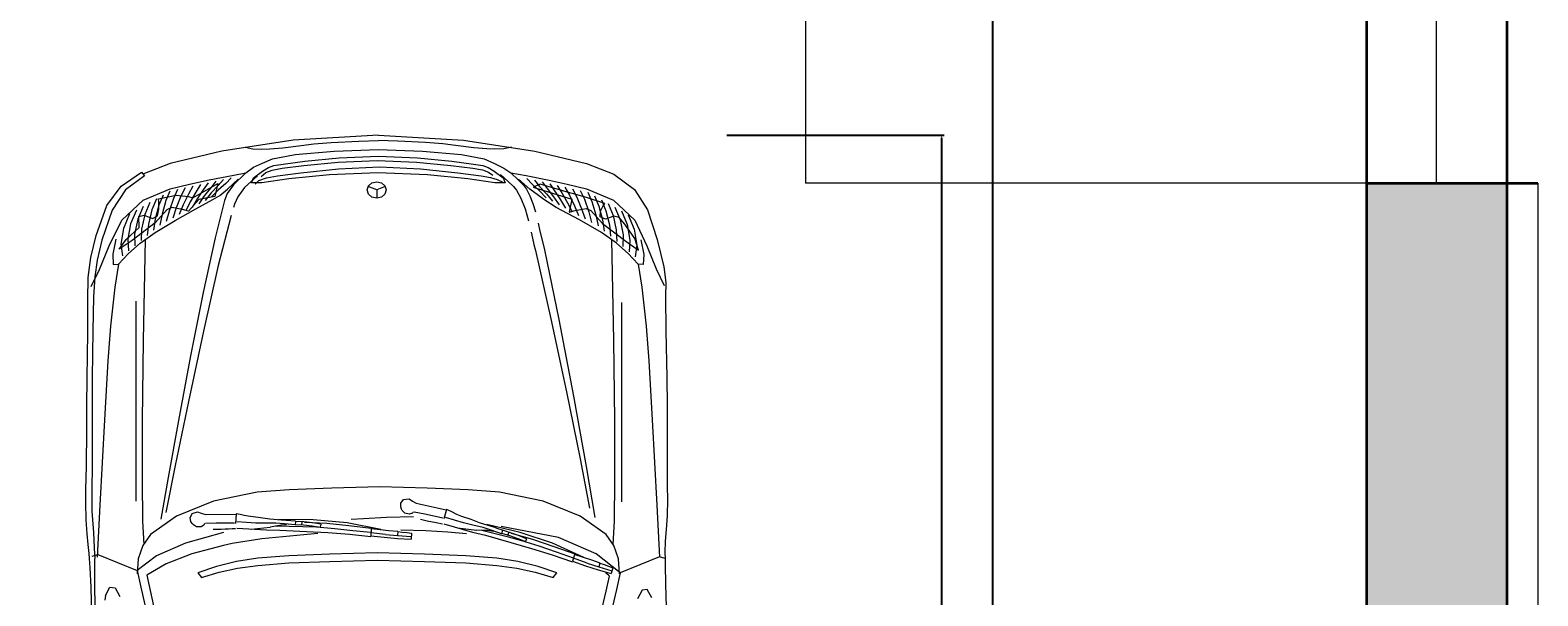
# Model space of a CAD drawing. Units: inches. Extents: x 37 to 706, y -568 to 110.
# Tile 6 of 24: x 126 to 223, y -378 to -342. Entities that reach past the tile are written whole.
import ezdxf

# ---------------------------------------------------------------- set-up
doc = ezdxf.new("R2010")
doc.units = ezdxf.units.IN
doc.header["$MEASUREMENT"] = 0
for name, color, linetype, lineweight in [('A-ANNO-DIMS', 2, 'Continuous', 18), ('A-DOOR', 4, 'Continuous', 18), ('A-FLOR-STRS', 7, 'Continuous', 18), ('A-GLAZ', 4, 'Continuous', 18), ('A-SITE-VEHI', 8, 'Continuous', 13), ('A-WALL', 7, 'Continuous', 35), ('A-WALL-PATT', 252, 'Continuous', 13)]:
    doc.layers.add(name, color=color, linetype=linetype, lineweight=lineweight)
doc.styles.get("Standard").update_dxf_attribs({"font": 'arial.ttf'})
doc.dimstyles.get("Standard").update_dxf_attribs({"dimtxt": 0.18, "dimasz": 0.18, "dimexe": 0.18, "dimexo": 0.0625, "dimgap": 0.09, "dimtad": 0, "dimtih": 1, "dimtoh": 1, "dimdec": 0, "dimzin": 0, "dimdsep": 46, "dimlunit": 3, "dimtxsty": 'Standard', "dimcen": 0.09, "dimadec": 0, "dimazin": 0, "dimtfac": 1, "dimtdec": 0, "dimtofl": 0, "dimtmove": 0, "dimatfit": 3, "dimfxl": 1, "dimtolj": 1, "dimtzin": 0, "dimarcsym": 0})

# ---------------------------------------------------------------- blocks, each defined once
blk = doc.blocks.new('CAR-SEDAN-PLAN')
for p, q in [((22.11, 92.169), (16.648, 91.844)), ((22.11, 92.169), (27.571, 91.844)), ((12.074, 91.146), (8.74, 90.335)), ((16.648, 91.844), (12.074, 91.146)), ((13.57, 91.383), (14.057, 91.284)), ((14.057, 91.284), (14.632, 91.256)), ((14.632, 91.256), (15.142, 91.276)), ((15.142, 91.276), (15.977, 91.359)), ((15.977, 91.359), (17.154, 91.49)), ((16.772, 90.917), (19.278, 91.146)), ((17.154, 91.49), (17.965, 91.597)), ((17.965, 91.597), (19.087, 91.685)), ((19.087, 91.685), (20.868, 91.772)), ((19.278, 91.146), (22.11, 91.24)), ((20.868, 91.772), (22.11, 91.812)), ((23.351, 91.772), (22.11, 91.812)), ((22.11, 91.24), (24.942, 91.146)), ((25.132, 91.685), (23.351, 91.772)), ((24.942, 91.146), (27.448, 90.917)), ((26.254, 91.597), (25.132, 91.685)), ((27.066, 91.49), (26.254, 91.597)), ((28.242, 91.359), (27.066, 91.49)), ((27.571, 91.844), (32.145, 91.146)), ((29.077, 91.276), (28.242, 91.359)), ((29.588, 91.256), (29.077, 91.276)), ((30.162, 91.284), (29.588, 91.256)), ((30.649, 91.383), (30.162, 91.284)), ((32.145, 91.146), (35.48, 90.335)), ((8.74, 90.335), (6.996, 89.668)), ((13.606, 89.739), (14.1, 90.1)), ((14.1, 90.1), (14.675, 90.37)), ((14.675, 90.37), (15.321, 90.633)), ((14.678, 89.847), (15.057, 90.081)), ((15.057, 90.081), (15.401, 90.212)), ((15.292, 89.924), (15.945, 90.036)), ((15.321, 90.633), (16.772, 90.917)), ((15.401, 90.212), (16, 90.311)), ((15.945, 90.036), (17.338, 90.213)), ((16, 90.311), (17.394, 90.488)), ((17.142, 89.744), (19.563, 89.998)), ((17.338, 90.213), (19.542, 90.43)), ((17.394, 90.488), (19.597, 90.705)), ((19.542, 90.43), (22.055, 90.536)), ((19.563, 89.998), (22.192, 90.123)), ((19.597, 90.705), (22.11, 90.811)), ((22.055, 90.536), (24.568, 90.43)), ((22.11, 90.811), (24.623, 90.705)), ((22.192, 90.123), (24.809, 89.998)), ((24.568, 90.43), (26.771, 90.213)), ((24.623, 90.705), (26.826, 90.488)), ((24.809, 89.998), (27.204, 89.744)), ((26.771, 90.213), (28.165, 90.036)), ((26.826, 90.488), (28.22, 90.311)), ((27.448, 90.917), (28.898, 90.633)), ((28.165, 90.036), (28.798, 89.928)), ((28.22, 90.311), (28.818, 90.212)), ((28.818, 90.212), (29.163, 90.081)), ((28.898, 90.633), (29.564, 90.343)), ((29.163, 90.081), (29.542, 89.847)), ((29.564, 90.343), (30.157, 90.045)), ((30.157, 90.045), (30.614, 89.739)), ((35.48, 90.335), (37.224, 89.668)), ((5.601, 88.894), (6.92, 89.795)), ((7.094, 89.544), (5.88, 88.648)), ((6.92, 89.795), (7.094, 89.544)), ((8.748, 88.708), (9.997, 89.025)), ((9.997, 89.025), (11.251, 89.289)), ((10.205, 88.137), (11.803, 89.066)), ((11.184, 89.102), (10.876, 88.651)), ((11.251, 89.289), (12.829, 89.594)), ((11.675, 89.21), (11.356, 88.789)), ((11.803, 89.066), (11.608, 88.22)), ((12.166, 89.318), (11.835, 88.927)), ((12.315, 89.065), (11.843, 88.651)), ((12.657, 89.426), (12.315, 89.065)), ((12.434, 88.691), (13.106, 89.346)), ((13.606, 89.739), (12.814, 88.982)), ((12.829, 89.594), (13.606, 89.739)), ((14.353, 89.555), (13.524, 88.797)), ((13.977, 89.1), (14.105, 89.414)), ((14.642, 89.096), (13.977, 89.1)), ((14.105, 89.414), (14.678, 89.847)), ((14.202, 89.012), (14.451, 89.242)), ((14.451, 89.242), (14.927, 89.418)), ((14.587, 89.505), (14.885, 89.766)), ((16.373, 89.358), (14.642, 89.096)), ((14.885, 89.766), (15.292, 89.924)), ((14.927, 89.418), (15.632, 89.546)), ((15.632, 89.546), (17.142, 89.744)), ((18.969, 89.62), (16.373, 89.358)), ((22.074, 89.739), (18.969, 89.62)), ((21.485, 88.91), (21.701, 89.101)), ((21.701, 89.101), (22.006, 89.174)), ((22.006, 89.174), (22.31, 89.101)), ((25.258, 89.62), (22.074, 89.739)), ((22.31, 89.101), (22.527, 88.91)), ((27.858, 89.358), (25.258, 89.62)), ((27.204, 89.744), (28.701, 89.546)), ((29.577, 89.096), (27.858, 89.358)), ((28.701, 89.546), (29.312, 89.449)), ((28.798, 89.928), (29.18, 89.791)), ((29.18, 89.791), (29.461, 89.588)), ((29.312, 89.449), (29.741, 89.324)), ((29.542, 89.847), (30.115, 89.414)), ((30.243, 89.1), (29.577, 89.096)), ((29.741, 89.324), (30.104, 89.134)), ((29.953, 89.642), (30.45, 89.191)), ((30.115, 89.414), (30.243, 89.1)), ((30.45, 89.191), (30.787, 88.865)), ((30.614, 89.739), (31.103, 89.28)), ((30.614, 89.739), (31.589, 89.567)), ((31.103, 89.28), (31.434, 88.948)), ((31.832, 88.694), (31.114, 89.346)), ((31.589, 89.567), (33.068, 89.276)), ((31.634, 89.371), (31.976, 89.009)), ((32.125, 89.263), (32.456, 88.872)), ((32.616, 89.155), (32.935, 88.733)), ((33.068, 89.276), (34.222, 89.025)), ((33.107, 89.047), (33.415, 88.595)), ((34.222, 89.025), (35.471, 88.708)), ((37.224, 89.668), (38.558, 88.671)), ((4.688, 87.635), (5.601, 88.894)), ((5.88, 88.648), (5.034, 87.338)), ((7.007, 87.995), (8.748, 88.708)), ((7.869, 88.075), (7.573, 87.365)), ((8.004, 88.083), (9.141, 88.312)), ((8.018, 87.864), (8.004, 88.083)), ((8.299, 88.318), (8.025, 87.663)), ((8.729, 88.56), (8.478, 87.96)), ((8.958, 88.098), (8.681, 87.291)), ((9.22, 88.669), (8.958, 88.098)), ((9.438, 88.236), (9.133, 87.485)), ((9.141, 88.312), (9.918, 88.231)), ((9.711, 88.777), (9.438, 88.236)), ((9.917, 88.374), (9.585, 87.68)), ((10.202, 88.885), (9.917, 88.374)), ((9.918, 88.231), (10.205, 88.137)), ((10.397, 88.512), (10.036, 87.874)), ((10.488, 88.068), (10.162, 87.52)), ((10.693, 88.993), (10.397, 88.512)), ((10.876, 88.651), (10.488, 88.068)), ((10.94, 88.262), (10.579, 87.747)), ((11.608, 88.22), (10.59, 88.027)), ((11.356, 88.789), (10.94, 88.262)), ((11.391, 88.457), (10.996, 87.974)), ((11.835, 88.927), (11.391, 88.457)), ((11.843, 88.651), (11.413, 88.201)), ((11.498, 88.024), (11.93, 88.29)), ((11.93, 88.29), (12.434, 88.691)), ((12.414, 88.426), (12.237, 87.977)), ((12.814, 88.982), (12.414, 88.426)), ((13.084, 88.202), (12.881, 87.731)), ((13.524, 88.797), (13.084, 88.202)), ((21.403, 88.642), (21.485, 88.91)), ((21.485, 88.373), (21.403, 88.642)), ((22.006, 88.642), (21.465, 88.872)), ((21.701, 88.182), (21.485, 88.373)), ((22.006, 88.11), (21.701, 88.182)), ((22.546, 88.872), (22.006, 88.642)), ((22.006, 88.642), (22.006, 88.11)), ((22.31, 88.182), (22.006, 88.11)), ((22.527, 88.373), (22.31, 88.182)), ((22.527, 88.91), (22.609, 88.642)), ((22.609, 88.642), (22.527, 88.373)), ((30.787, 88.865), (30.971, 88.623)), ((30.971, 88.623), (31.247, 88.111)), ((31.247, 88.111), (31.528, 87.423)), ((31.434, 88.948), (31.614, 88.703)), ((31.614, 88.703), (31.841, 88.274)), ((32.384, 88.296), (31.832, 88.694)), ((31.841, 88.274), (32.036, 87.783)), ((31.976, 89.009), (32.448, 88.596)), ((32.488, 89.011), (32.052, 88.817)), ((32.052, 88.817), (34.523, 88.059)), ((32.722, 88.024), (32.384, 88.296)), ((32.448, 88.596), (32.878, 88.146)), ((32.456, 88.872), (32.9, 88.401)), ((34.313, 88.478), (32.488, 89.011)), ((32.9, 88.401), (33.295, 87.919)), ((32.935, 88.733), (33.351, 88.207)), ((33.351, 88.207), (33.712, 87.692)), ((33.415, 88.595), (33.803, 88.013)), ((33.598, 88.938), (33.895, 88.457)), ((33.895, 88.457), (34.255, 87.819)), ((34.089, 88.83), (34.374, 88.319)), ((34.633, 88.402), (34.313, 88.478)), ((34.523, 88.059), (34.362, 87.218)), ((34.374, 88.319), (34.706, 87.625)), ((34.58, 88.722), (34.854, 88.181)), ((35.469, 88.167), (34.633, 88.402)), ((34.854, 88.181), (35.158, 87.43)), ((35.071, 88.613), (35.333, 88.043)), ((36.639, 87.768), (35.469, 88.167)), ((35.471, 88.708), (37.213, 87.995)), ((35.562, 88.505), (35.813, 87.905)), ((35.992, 88.263), (36.266, 87.608)), ((38.558, 88.671), (39.379, 87.367)), ((3.994, 85.722), (4.688, 87.635)), ((5.034, 87.338), (4.368, 85.408)), ((5.638, 86.702), (7.007, 87.995)), ((6.149, 87.105), (5.761, 86.175)), ((6.579, 87.348), (6.214, 86.472)), ((7.009, 87.59), (6.667, 86.77)), ((7.439, 87.833), (7.12, 87.067)), ((7.573, 87.365), (7.35, 86.452)), ((8.025, 87.663), (7.79, 86.774)), ((8.54, 87.37), (7.797, 86.541)), ((7.943, 86.98), (8.02, 87.4)), ((8.02, 87.4), (8.018, 87.864)), ((8.23, 87.097), (8.076, 86.385)), ((8.478, 87.96), (8.23, 87.097)), ((8.681, 87.291), (8.494, 86.612)), ((8.851, 87.516), (8.54, 87.37)), ((9.545, 87.384), (8.851, 87.516)), ((9.133, 87.485), (8.911, 86.839)), ((9.062, 86.674), (10.405, 87.423)), ((9.585, 87.68), (9.328, 87.066)), ((9.93, 87.273), (9.545, 87.384)), ((10.036, 87.874), (9.745, 87.293)), ((10.59, 88.027), (9.93, 87.273)), ((10.405, 87.423), (11.498, 88.024)), ((12.237, 87.977), (11.632, 85.572)), ((12.881, 87.731), (12.809, 87.511)), ((31.528, 87.423), (31.755, 86.658)), ((32.036, 87.783), (32.207, 87.242)), ((33.526, 87.525), (32.722, 88.024)), ((35.014, 86.725), (33.526, 87.525)), ((33.803, 88.013), (34.129, 87.465)), ((34.255, 87.819), (34.546, 87.238)), ((34.362, 87.218), (34.746, 87.329)), ((34.706, 87.625), (34.963, 87.011)), ((34.746, 87.329), (35.44, 87.461)), ((35.158, 87.43), (35.38, 86.784)), ((35.333, 88.043), (35.61, 87.236)), ((35.44, 87.461), (35.751, 87.315)), ((35.61, 87.236), (35.798, 86.557)), ((35.751, 87.315), (36.494, 86.486)), ((35.813, 87.905), (36.062, 87.042)), ((36.266, 87.608), (36.501, 86.719)), ((36.348, 86.925), (36.363, 87.278)), ((36.363, 87.278), (36.533, 87.617)), ((36.422, 88.02), (36.718, 87.31)), ((36.533, 87.617), (36.639, 87.768)), ((36.718, 87.31), (36.941, 86.397)), ((36.852, 87.778), (37.171, 87.012)), ((37.213, 87.995), (38.581, 86.702)), ((37.282, 87.535), (37.624, 86.715)), ((37.712, 87.293), (38.077, 86.417)), ((39.379, 87.367), (40.01, 85.452)), ((4.843, 85.044), (5.638, 86.702)), ((5.761, 86.175), (5.591, 85.161)), ((5.921, 85.456), (6.761, 86.233)), ((6.214, 86.472), (6.031, 85.483)), ((7.797, 86.541), (6.303, 85.406)), ((6.667, 86.77), (6.471, 85.806)), ((6.735, 86.931), (7.077, 87.019)), ((6.761, 86.233), (6.735, 86.931)), ((6.91, 86.129), (6.882, 85.394)), ((7.12, 87.067), (6.91, 86.129)), ((7.077, 87.019), (7.607, 86.812)), ((7.35, 86.452), (7.28, 85.724)), ((7.607, 86.812), (7.943, 86.98)), ((7.79, 86.774), (7.678, 86.054)), ((7.782, 85.916), (9.062, 86.674)), ((12.655, 87.001), (11.831, 83.79)), ((32.36, 86.52), (32.484, 85.989)), ((36.437, 85.916), (35.014, 86.725)), ((36.062, 87.042), (36.215, 86.33)), ((36.684, 86.757), (36.348, 86.925)), ((36.494, 86.486), (37.989, 85.351)), ((36.501, 86.719), (36.613, 85.999)), ((37.214, 86.963), (36.684, 86.757)), ((36.941, 86.397), (37.011, 85.669)), ((37.171, 87.012), (37.381, 86.074)), ((37.557, 86.876), (37.214, 86.963)), ((37.923, 86.436), (37.557, 86.876)), ((37.624, 86.715), (37.821, 85.751)), ((38.567, 85.53), (37.923, 86.436)), ((38.077, 86.417), (38.26, 85.428)), ((38.142, 87.05), (38.53, 86.12)), ((38.581, 86.702), (39.352, 85.06)), ((3.655, 84.305), (3.994, 85.722)), ((4.368, 85.408), (4.064, 84.126)), ((5.266, 85.479), (5.072, 84.518)), ((5.486, 84.834), (5.921, 85.456)), ((6.303, 85.406), (5.486, 84.834)), ((5.591, 85.161), (5.688, 84.402)), ((6.031, 85.483), (6.086, 84.733)), ((6.083, 84.566), (6.814, 85.229)), ((6.471, 85.806), (6.484, 85.063)), ((6.814, 85.229), (7.782, 85.916)), ((7.139, 85.452), (7.018, 78.984)), ((11.632, 85.572), (10.878, 82.065)), ((31.915, 85.932), (32.007, 85.538)), ((32.007, 85.538), (32.098, 85.143)), ((32.484, 85.989), (32.641, 85.34)), ((32.641, 85.34), (32.766, 84.808)), ((37.406, 85.229), (36.437, 85.916)), ((37.081, 85.452), (37.201, 78.984)), ((37.381, 86.074), (37.409, 85.339)), ((38.137, 84.566), (37.406, 85.229)), ((37.821, 85.751), (37.807, 85.008)), ((37.989, 85.351), (38.805, 84.779)), ((38.26, 85.428), (38.205, 84.678)), ((38.53, 86.12), (38.7, 85.105)), ((38.805, 84.779), (38.567, 85.53)), ((38.964, 85.445), (39.149, 84.498)), ((40.01, 85.452), (40.443, 83.712)), ((3.488, 83.013), (3.655, 84.305)), ((4.207, 83.537), (4.843, 85.044)), ((5.072, 84.518), (5.102, 83.849)), ((5.424, 83.88), (6.083, 84.566)), ((32.098, 85.143), (32.191, 84.749)), ((32.191, 84.749), (33.187, 80.374)), ((32.766, 84.808), (33.695, 80.324)), ((38.796, 83.88), (38.137, 84.566)), ((38.7, 85.105), (38.604, 84.347)), ((39.149, 84.498), (39.115, 83.845)), ((39.352, 85.06), (39.944, 83.583)), ((3.673, 82.45), (4.207, 83.537)), ((4.064, 84.126), (3.924, 83.058)), ((5.102, 83.849), (5.424, 83.88)), ((5.424, 83.88), (5.2, 82.403)), ((11.831, 83.79), (10.879, 79.575)), ((38.796, 83.88), (39.019, 82.403)), ((39.115, 83.845), (38.796, 83.88)), ((39.944, 83.583), (40.454, 82.512)), ((40.443, 83.712), (40.566, 82.702)), ((3.471, 81.595), (3.488, 83.013)), ((3.924, 83.058), (3.838, 81.777)), ((5.2, 82.403), (4.921, 79.902)), ((39.019, 82.403), (39.298, 79.902)), ((40.566, 82.702), (40.546, 81.772)), ((3.469, 79.46), (3.471, 81.595)), ((3.838, 81.777), (3.783, 79.595)), ((6.575, 68.65), (6.575, 81.495)), ((10.878, 82.065), (10.063, 77.979)), ((37.735, 68.611), (37.735, 81.405)), ((40.546, 81.772), (40.558, 79.591)), ((33.187, 80.374), (34.19, 75.667)), ((33.695, 80.324), (34.635, 75.398)), ((3.427, 76.546), (3.469, 79.46)), ((3.783, 79.595), (3.753, 76.594)), ((4.921, 79.902), (4.745, 77.663)), ((10.879, 79.575), (9.92, 75.059)), ((39.298, 79.902), (39.474, 77.663)), ((40.558, 79.591), (40.618, 76.592)), ((7.018, 78.984), (6.954, 73.857)), ((37.201, 78.984), (37.265, 73.857)), ((4.745, 77.663), (4.545, 73.869)), ((10.063, 77.979), (9.279, 73.84)), ((39.474, 77.663), (39.674, 73.869)), ((3.401, 74.768), (3.427, 76.546)), ((3.753, 76.594), (3.743, 74.768)), ((40.618, 76.592), (40.653, 74.768)), ((34.19, 75.667), (35.061, 71.363)), ((3.394, 73.244), (3.401, 74.768)), ((3.743, 74.768), (3.745, 73.25)), ((9.92, 75.059), (9.08, 70.94)), ((34.635, 75.398), (35.451, 70.877)), ((40.653, 74.768), (40.646, 73.29)), ((4.545, 73.869), (4.242, 68.391)), ((6.954, 73.857), (6.943, 70.006)), ((9.279, 73.84), (8.614, 70.171)), ((37.265, 73.857), (37.276, 70.006)), ((39.674, 73.869), (39.977, 68.391)), ((3.374, 70.909), (3.394, 73.244)), ((3.745, 73.25), (3.741, 70.929)), ((40.646, 73.29), (40.638, 71.042)), ((3.343, 69.409), (3.374, 70.909)), ((3.741, 70.929), (3.719, 69.434)), ((9.08, 70.94), (8.479, 67.921)), ((35.061, 71.363), (35.662, 68.196)), ((35.451, 70.877), (36.007, 67.608)), ((40.638, 71.042), (40.653, 69.588)), ((6.943, 70.006), (6.982, 67.366)), ((8.614, 70.171), (8.158, 67.498)), ((37.276, 70.006), (37.237, 67.366)), ((3.33, 68.57), (3.343, 69.409)), ((3.719, 69.434), (3.721, 68.015)), ((14.339, 69.23), (11.529, 68.645)), ((16.386, 69.388), (14.339, 69.23)), ((19.12, 69.493), (16.386, 69.388)), ((22.208, 69.572), (19.12, 69.493)), ((25.245, 69.493), (22.208, 69.572)), ((23.551, 68.52), (23.735, 68.76)), ((23.735, 68.76), (24.097, 68.799)), ((24.097, 68.799), (24.299, 68.657)), ((27.884, 69.388), (25.245, 69.493)), ((29.881, 69.23), (27.884, 69.388)), ((32.691, 68.645), (29.881, 69.23)), ((40.667, 68.779), (40.64, 67.717)), ((40.653, 69.588), (40.667, 68.779)), ((3.357, 67.456), (3.33, 68.57)), ((3.721, 68.015), (3.826, 66.632)), ((4.242, 68.391), (4.066, 65.05)), ((11.529, 68.645), (9.151, 67.695)), ((10.038, 67.577), (10.163, 67.852)), ((10.163, 67.852), (10.507, 67.971)), ((10.507, 67.971), (10.736, 67.879)), ((10.736, 67.879), (11.007, 67.807)), ((11.007, 67.807), (12.981, 67.817)), ((12.984, 67.849), (12.948, 67.224)), ((13.239, 67.799), (12.984, 67.849)), ((13.505, 67.735), (13.239, 67.799)), ((13.761, 67.687), (13.505, 67.735)), ((23.545, 68.289), (23.551, 68.52)), ((23.59, 68.141), (23.545, 68.289)), ((23.648, 68.043), (23.59, 68.141)), ((23.818, 67.872), (23.648, 68.043)), ((24.099, 67.811), (23.818, 67.872)), ((24.296, 67.875), (24.099, 67.811)), ((24.325, 67.935), (24.296, 67.875)), ((24.299, 68.657), (24.546, 68.526)), ((24.361, 67.962), (24.325, 67.935)), ((25.085, 67.81), (24.416, 67.948)), ((24.546, 68.526), (26.473, 68.092)), ((25.584, 67.703), (25.085, 67.81)), ((26.483, 68.122), (26.307, 67.522)), ((26.786, 67.983), (26.483, 68.122)), ((27.155, 67.801), (26.786, 67.983)), ((27.463, 67.673), (27.155, 67.801)), ((35.069, 67.695), (32.691, 68.645)), ((39.977, 68.391), (40.153, 65.05)), ((3.416, 66.545), (3.357, 67.456)), ((6.982, 67.366), (7.068, 65.872)), ((9.151, 67.695), (7.496, 66.515)), ((10.084, 67.351), (10.038, 67.577)), ((10.162, 67.216), (10.084, 67.351)), ((10.239, 67.134), (10.162, 67.216)), ((10.444, 67.005), (10.239, 67.134)), ((10.732, 67.009), (10.444, 67.005)), ((10.909, 67.115), (10.732, 67.009)), ((10.924, 67.181), (10.909, 67.115)), ((10.952, 67.215), (10.924, 67.181)), ((11.692, 67.23), (11.009, 67.214)), ((11.499, 66.856), (11.754, 66.85)), ((12.202, 67.238), (11.692, 67.23)), ((11.754, 66.85), (12.013, 66.864)), ((12.013, 66.864), (12.269, 66.878)), ((12.885, 67.248), (12.202, 67.238)), ((12.269, 66.878), (12.494, 66.885)), ((12.494, 66.885), (12.72, 66.89)), ((12.72, 66.89), (12.945, 66.9)), ((13.035, 66.911), (14.939, 66.803)), ((13.653, 67.289), (13.037, 67.33)), ((14.246, 67.249), (13.653, 67.289)), ((14.556, 67.58), (13.761, 67.687)), ((13.945, 66.863), (15.177, 66.982)), ((14.864, 67.243), (14.246, 67.249)), ((15.155, 67.5), (14.556, 67.58)), ((15.54, 67.244), (14.864, 67.243)), ((14.939, 66.803), (15.789, 66.795)), ((15.898, 67.437), (15.155, 67.5)), ((15.525, 67.047), (15.177, 66.982)), ((16.386, 67.022), (15.503, 67.047)), ((15.873, 67.117), (15.525, 67.047)), ((16.088, 67.199), (15.54, 67.244)), ((17.922, 67.462), (15.723, 67.48)), ((15.789, 66.795), (16.643, 66.752)), ((16.224, 67.141), (15.873, 67.117)), ((16.194, 67.415), (15.898, 67.437)), ((16.776, 67.124), (16.088, 67.199)), ((16.497, 67.388), (16.194, 67.415)), ((17.269, 67.011), (16.386, 67.022)), ((16.792, 67.365), (16.497, 67.388)), ((16.766, 67.163), (17.31, 67.127)), ((16.797, 67.346), (16.776, 67.124)), ((17.329, 67.319), (16.785, 67.353)), ((17.204, 67.326), (17.186, 67.136)), ((18.152, 66.977), (17.269, 67.011)), ((17.31, 67.127), (17.856, 67.065)), ((17.876, 67.251), (17.329, 67.319)), ((17.365, 67.301), (18.795, 67.235)), ((17.856, 67.065), (18.396, 66.992)), ((18.416, 67.172), (17.876, 67.251)), ((20.11, 67.269), (17.922, 67.462)), ((19.315, 66.878), (18.152, 66.977)), ((18.416, 67.172), (18.386, 66.99)), ((18.795, 67.235), (20.227, 67.083)), ((20.476, 66.753), (19.315, 66.878)), ((22.264, 66.832), (20.11, 67.269)), ((20.227, 67.083), (21.653, 66.928)), ((21.152, 67.521), (20.364, 67.481)), ((22.637, 67.604), (21.152, 67.521)), ((21.653, 66.928), (21.624, 66.426)), ((21.652, 66.887), (22.219, 66.829)), ((22.219, 66.829), (22.786, 66.779)), ((24.36, 67.655), (22.637, 67.604)), ((22.786, 66.779), (23.353, 66.722)), ((25.16, 66.751), (23.552, 66.78)), ((24.813, 67.489), (25.236, 67.39)), ((25.236, 67.39), (25.817, 67.28)), ((26.251, 67.559), (25.584, 67.703)), ((25.817, 67.28), (26.231, 67.207)), ((26.322, 67.197), (28.153, 66.664)), ((27.008, 67.427), (26.417, 67.605)), ((27.578, 67.254), (27.008, 67.427)), ((27.197, 66.945), (28.425, 66.784)), ((28.075, 67.467), (27.463, 67.673)), ((28.178, 67.109), (27.578, 67.254)), ((28.604, 67.264), (28.075, 67.467)), ((28.837, 66.958), (28.178, 67.109)), ((28.778, 66.769), (28.425, 66.784)), ((29.229, 67.066), (28.604, 67.264)), ((29.611, 66.552), (28.756, 66.774)), ((29.133, 66.759), (28.778, 66.769)), ((29.361, 66.791), (28.837, 66.958)), ((31.207, 66.635), (29.068, 67.147)), ((29.514, 66.981), (29.229, 67.066)), ((30.014, 66.563), (29.361, 66.791)), ((29.802, 66.885), (29.514, 66.981)), ((30.085, 66.794), (29.802, 66.885)), ((33.664, 66.317), (29.991, 67.029)), ((30.085, 66.774), (30.014, 66.563)), ((30.597, 66.628), (30.074, 66.784)), ((36.723, 66.515), (35.069, 67.695)), ((37.237, 67.366), (37.152, 65.872)), ((40.582, 66.836), (40.524, 66.091)), ((40.64, 67.717), (40.582, 66.836)), ((3.49, 65.874), (3.416, 66.545)), ((3.553, 65.288), (3.49, 65.874)), ((3.826, 66.632), (3.887, 65.216)), ((6.998, 65.803), (6.705, 64.942)), ((7.496, 66.515), (6.998, 65.803)), ((9.728, 65.963), (7.877, 65.137)), ((12.165, 66.636), (9.728, 65.963)), ((12.165, 65.811), (10.134, 65.275)), ((12.721, 65.94), (12.165, 65.811)), ((14.625, 66.238), (12.721, 65.94)), ((18.234, 66.568), (14.625, 66.238)), ((16.643, 66.752), (17.493, 66.701)), ((17.493, 66.701), (18.865, 66.631)), ((18.865, 66.631), (20.259, 66.538)), ((20.259, 66.538), (21.624, 66.384)), ((21.638, 66.636), (20.476, 66.753)), ((21.624, 66.426), (22.487, 66.333)), ((22.566, 66.509), (21.631, 66.624)), ((22.487, 66.333), (23.347, 66.265)), ((22.566, 66.509), (23.333, 66.449)), ((23.357, 66.702), (23.333, 66.449)), ((23.333, 66.449), (24.216, 66.384)), ((23.347, 66.265), (24.213, 66.218)), ((23.357, 66.702), (23.648, 66.671)), ((23.648, 66.671), (23.94, 66.635)), ((23.94, 66.635), (24.229, 66.594)), ((24.229, 66.594), (24.213, 66.218)), ((26.574, 66.668), (25.16, 66.751)), ((27.773, 66.553), (26.574, 66.668)), ((28.153, 66.664), (28.979, 66.465)), ((28.979, 66.465), (29.801, 66.23)), ((29.481, 66.704), (29.133, 66.759)), ((30.469, 66.342), (29.611, 66.552)), ((29.801, 66.23), (30.618, 65.99)), ((30.014, 66.603), (30.535, 66.446)), ((30.477, 66.664), (30.416, 66.483)), ((31.322, 66.11), (30.469, 66.342)), ((30.535, 66.446), (31.054, 66.263)), ((31.115, 66.439), (30.597, 66.628)), ((30.618, 65.99), (31.939, 65.612)), ((30.628, 66.603), (32.006, 66.218)), ((31.054, 66.263), (31.563, 66.07)), ((31.624, 66.241), (31.115, 66.439)), ((33.296, 65.954), (31.207, 66.635)), ((32.433, 65.752), (31.322, 66.11)), ((31.624, 66.241), (31.553, 66.07)), ((32.006, 66.218), (33.368, 65.747)), ((35.296, 65.044), (33.296, 65.954)), ((36.098, 65.263), (33.664, 66.317)), ((37.222, 65.803), (36.723, 66.515)), ((37.515, 64.942), (37.222, 65.803)), ((40.524, 66.091), (40.497, 65.354)), ((3.583, 64.975), (3.553, 65.288)), ((3.614, 64.361), (3.583, 64.975)), ((3.746, 65.115), (4.101, 65.222)), ((3.887, 65.216), (3.9, 65.188)), ((3.9, 65.188), (3.908, 65.155)), ((3.911, 65.118), (3.903, 64.803)), ((3.908, 65.155), (3.911, 65.118)), ((4.101, 65.222), (6.623, 64.191)), ((7.877, 65.137), (6.623, 64.191)), ((6.705, 64.942), (6.639, 63.978)), ((10.134, 65.275), (8.491, 64.633)), ((14.37, 64.993), (13.014, 64.773)), ((16.366, 65.151), (14.37, 64.993)), ((19.006, 65.255), (16.366, 65.151)), ((22.043, 65.335), (19.006, 65.255)), ((19.006, 64.788), (22.043, 64.867)), ((25.08, 65.255), (22.043, 65.335)), ((22.043, 64.867), (25.08, 64.788)), ((27.719, 65.151), (25.08, 65.255)), ((29.716, 64.993), (27.719, 65.151)), ((31.072, 64.773), (29.716, 64.993)), ((31.939, 65.612), (33.276, 65.209)), ((33.537, 65.369), (32.433, 65.752)), ((33.276, 65.209), (34.572, 64.752)), ((33.368, 65.747), (34.723, 65.275)), ((34.642, 64.993), (33.537, 65.369)), ((34.723, 65.275), (34.582, 64.792)), ((35.517, 64.662), (34.632, 64.983)), ((34.713, 65.235), (35.252, 65.051)), ((35.252, 65.051), (35.793, 64.875)), ((35.793, 64.875), (36.332, 64.692)), ((37.632, 64.039), (36.098, 65.263)), ((37.581, 63.978), (37.515, 64.942)), ((40.154, 65.07), (37.632, 64.039)), ((40.509, 64.963), (40.154, 65.07)), ((40.497, 65.354), (40.511, 64.943)), ((40.511, 64.943), (40.516, 64.555)), ((3.672, 63.126), (3.614, 64.361)), ((3.903, 64.803), (3.894, 63.679)), ((6.623, 64.191), (6.866, 63.136)), ((8.491, 64.633), (7.243, 63.902)), ((7.243, 63.902), (9.479, 53.69)), ((11.719, 64.455), (10.517, 64.056)), ((10.517, 64.056), (10.762, 63.739)), ((10.762, 63.739), (11.901, 64.099)), ((13.014, 64.773), (11.719, 64.455)), ((11.901, 64.099), (13.077, 64.344)), ((13.077, 64.344), (14.37, 64.526)), ((14.37, 64.526), (16.366, 64.684)), ((16.366, 64.684), (19.006, 64.788)), ((25.08, 64.788), (27.719, 64.684)), ((27.719, 64.684), (29.716, 64.526)), ((29.716, 64.526), (31.008, 64.344)), ((31.008, 64.344), (32.184, 64.099)), ((32.366, 64.455), (31.072, 64.773)), ((32.184, 64.099), (33.323, 63.739)), ((33.569, 64.056), (32.366, 64.455)), ((33.323, 63.739), (33.569, 64.056)), ((34.582, 64.792), (35.401, 64.507)), ((35.401, 64.507), (36.224, 64.248)), ((35.517, 64.662), (36.252, 64.43)), ((36.224, 64.248), (37.057, 64.008)), ((36.332, 64.672), (36.252, 64.43)), ((36.252, 64.43), (37.097, 64.168)), ((36.332, 64.672), (36.609, 64.576)), ((36.609, 64.576), (36.884, 64.475)), ((36.79, 63.963), (36.704, 64.018)), ((36.874, 63.902), (36.79, 63.963)), ((36.956, 63.837), (36.874, 63.902)), ((36.884, 64.475), (37.157, 64.37)), ((37.157, 64.37), (37.057, 64.008)), ((37.632, 64.039), (37.389, 62.984)), ((40.516, 64.555), (40.544, 63.318)), ((3.719, 61.318), (3.672, 63.126)), ((3.894, 63.679), (3.912, 61.483)), ((4.598, 62.593), (4.885, 63.135)), ((4.885, 63.135), (5.211, 63.093)), ((5.211, 63.093), (5.522, 62.522)), ((6.866, 63.136), (7.386, 60.866)), ((36.731, 62.877), (36.956, 63.837)), ((37.389, 62.984), (36.869, 60.714)), ((39.044, 62.941), (38.733, 62.37)), ((39.37, 62.983), (39.044, 62.941)), ((39.657, 62.441), (39.37, 62.983)), ((40.544, 63.318), (40.611, 61.119)), ((4.598, 62.593), (4.555, 62.29)), ((36.246, 60.784), (36.731, 62.877))]:
    blk.add_line(p, q)
blk = doc.blocks.new('*D29')
at = {"layer": 'A-ANNO-DIMS', "color": 0, "lineweight": -2, "transparency": 16777216}
for p, q in [((170.913, -348.62), (184.856, -348.62)), ((184.676, -348.8), (184.676, -394.522)), ((184.676, -440.609), (184.676, -394.888)), ((170.913, -440.789), (184.856, -440.789))]:
    blk.add_line(p, q, dxfattribs=at)
at = {"layer": 'A-ANNO-DIMS', "color": 0, "transparency": 16777216}
for points in [[(184.646, -348.8), (184.706, -348.8), (184.676, -348.62)], [(184.646, -440.609), (184.706, -440.609), (184.676, -440.789)]]:
    blk.add_solid(points, dxfattribs=at)
at = {"layer": 'Defpoints', "color": 0, "transparency": 16777216}
for p in [(170.851, -348.62), (184.676, -348.62), (170.851, -440.789)]:
    blk.add_point(p, dxfattribs=at)
at = {"layer": 'A-ANNO-DIMS', "color": 0, "transparency": 16777216, "insert": (184.676, -394.705), "char_height": 0.18, "attachment_point": 5}
blk.add_mtext('\\A1;CAR 7\'-8" TYP.', dxfattribs=at)
blk = doc.blocks.new('*D51')
at = {"layer": 'A-ANNO-DIMS', "color": 0, "lineweight": -2, "transparency": 16777216}
for p, q in [((220.958, -294.771), (220.958, -567.638)), ((251.958, -294.771), (251.958, -567.638)), ((221.138, -567.458), (236.128, -567.458)), ((251.778, -567.458), (236.789, -567.458))]:
    blk.add_line(p, q, dxfattribs=at)
at = {"layer": 'A-ANNO-DIMS', "color": 0, "transparency": 16777216}
for points in [[(221.138, -567.428), (221.138, -567.488), (220.958, -567.458)], [(251.778, -567.428), (251.778, -567.488), (251.958, -567.458)]]:
    blk.add_solid(points, dxfattribs=at)
at = {"layer": 'Defpoints', "color": 0, "transparency": 16777216}
for p in [(220.958, -294.708), (251.958, -294.708), (251.958, -567.458)]:
    blk.add_point(p, dxfattribs=at)
at = {"layer": 'A-ANNO-DIMS', "color": 0, "transparency": 16777216, "insert": (236.458, -567.458), "char_height": 0.18, "attachment_point": 5}
blk.add_mtext('\\A1;2\'-7"', dxfattribs=at)
blk = doc.blocks.new('*D62')
at = {"layer": 'A-ANNO-DIMS', "color": 0, "lineweight": -2, "transparency": 16777216}
for p, q in [((187.958, -142.771), (187.958, -567.638)), ((211.958, -142.771), (211.958, -567.638)), ((188.138, -567.458), (199.628, -567.458)), ((211.778, -567.458), (200.289, -567.458))]:
    blk.add_line(p, q, dxfattribs=at)
at = {"layer": 'A-ANNO-DIMS', "color": 0, "transparency": 16777216}
for points in [[(188.138, -567.428), (188.138, -567.488), (187.958, -567.458)], [(211.778, -567.428), (211.778, -567.488), (211.958, -567.458)]]:
    blk.add_solid(points, dxfattribs=at)
at = {"layer": 'Defpoints', "color": 0, "transparency": 16777216}
for p in [(187.958, -142.708), (211.958, -142.708), (211.958, -567.458)]:
    blk.add_point(p, dxfattribs=at)
at = {"layer": 'A-ANNO-DIMS', "color": 0, "transparency": 16777216, "insert": (199.958, -567.458), "char_height": 0.18, "attachment_point": 5}
blk.add_mtext('\\A1;2\'-0"', dxfattribs=at)

msp = doc.modelspace()

# ---------------------------------------------------------------- hatches: boundary and pattern name
at = {"layer": 'A-WALL-PATT'}
h = msp.add_hatch(color=256, dxfattribs=at)
h.dxf.hatch_style = 1
h.paths.add_polyline_path([(220.958, -351.708), (211.958, -351.708), (211.958, -513.708), (254.958, -513.708), (254.958, -504.708), (220.958, -504.708)], flags=17)
h.paths.add_polyline_path([(220.958, -294.708), (211.958, -294.708), (211.958, -303.708), (220.958, -303.708)], flags=17)
h.paths.add_polyline_path([(175.958, -294.708), (155.871, -294.708), (155.871, -303.708), (155.958, -303.708), (175.958, -303.708)], flags=17)
h.paths.add_polyline_path([(220.958, -16.708), (211.958, -16.708), (211.958, -142.708), (220.958, -142.708)], flags=17)
h.paths.add_polyline_path([(357.958, 51.292), (78.958, 51.292), (78.958, -513.708), (87.958, -513.708), (87.958, -303.708), (95.871, -303.708), (95.871, -294.708), (87.958, -294.708), (87.958, -142.708), (187.958, -142.708), (187.958, -133.708), (87.958, -133.708), (87.958, -25.708), (106.958, -25.708), (106.958, -16.708), (87.958, -16.708), (87.958, 42.292), (348.958, 42.292), (348.958, 17.129), (348.958, -133.708), (246.958, -133.708), (246.958, -142.708), (348.958, -142.708), (348.958, -294.708), (251.958, -294.708), (251.958, -303.708), (348.958, -303.708), (348.958, -351.708), (260.958, -351.708), (260.958, -329.708), (251.958, -329.708), (251.958, -360.708), (327.446, -360.708), (348.958, -360.708), (348.958, -504.708), (314.958, -504.708), (314.958, -513.708), (357.958, -513.708)])
h.paths.add_polyline_path([(416.958, -303.708), (402.958, -303.708), (402.958, -151.708), (478.958, -151.708), (478.958, -142.708), (402.958, -142.708), (402.958, -22.708), (409.958, -22.708), (409.958, -13.708), (402.958, -13.708), (402.958, 42.292), (663.958, 42.292), (663.958, -303.708), (566.958, -303.708), (566.958, -312.708), (663.958, -312.708), (663.958, -360.708), (575.958, -360.708), (575.958, -338.708), (566.958, -338.708), (566.958, -360.708), (566.958, -369.708), (642.446, -369.708), (663.958, -369.708), (663.958, -513.708), (629.958, -513.708), (629.958, -522.708), (672.958, -522.708), (672.958, 51.292), (393.958, 51.292), (393.958, -522.708), (402.958, -522.708), (402.958, -312.708), (416.958, -312.708)])
h.paths.add_polyline_path([(490.958, -303.708), (476.958, -303.708), (476.958, -312.708), (490.958, -312.708)], flags=17)
h.paths.add_polyline_path([(535.958, -303.708), (526.958, -303.708), (526.958, -312.708), (535.958, -312.708)], flags=17)
h.paths.add_polyline_path([(535.958, -369.708), (526.958, -369.708), (526.958, -522.708), (569.958, -522.708), (569.958, -513.708), (535.958, -513.708)], flags=17)
h.paths.add_polyline_path([(511.958, -13.708), (502.958, -13.708), (502.958, -151.708), (511.958, -151.708)], flags=17)
h.paths.add_polyline_path([(651.539, -142.708), (651.539, -120.181), (642.539, -120.181), (642.539, -142.708), (550.539, -142.708), (550.539, -120.708), (541.539, -120.708), (541.539, -142.708), (537.958, -142.708), (537.958, -151.708), (651.539, -151.708)], flags=17)
h.paths.add_polyline_path([(651.539, -85.708), (541.539, -85.708), (541.539, -94.708), (651.539, -94.708)], flags=17)
h.paths.add_polyline_path([(476.958, -13.708), (469.958, -13.708), (469.958, -22.708), (476.958, -22.708)], flags=17)
h.paths.add_polyline_path([(185.958, -16.708), (166.958, -16.708), (166.958, -25.708), (185.958, -25.708)], flags=17)
h.paths.add_polyline_path([(168.909, -414.719), (214.621, -414.719), (214.621, -392.33), (168.909, -392.33)], flags=25)

# ---------------------------------------------------------------- linework, layer by layer
at = {"layer": 'A-DOOR'}
for p, q in [((222.958, -351.708), (222.958, -360.708)), ((222.958, -360.708), (222.958, -384.708))]:
    msp.add_line(p, q, dxfattribs=at)
at = {"layer": 'A-FLOR-STRS'}
for p in [(175.958, -303.708), (211.958, -351.708)]:
    msp.add_line(p, (175.958, -351.708), dxfattribs=at)
at = {"layer": 'A-GLAZ'}
msp.add_line((216.458, -351.708), (216.458, -303.708), dxfattribs=at)
at = {"layer": 'A-WALL'}
for p, q in [((211.958, -294.708), (211.958, -513.708)), ((220.958, -294.708), (220.958, -504.708)), ((211.958, -351.708), (220.958, -351.708)), ((220.958, -351.708), (222.958, -351.708))]:
    msp.add_line(p, q, dxfattribs=at)

# ---------------------------------------------------------------- block references
at = {"layer": 'A-SITE-VEHI'}
msp.add_blockref('CAR-SEDAN-PLAN', (126.431, -440.789), dxfattribs=at)

# ---------------------------------------------------------------- dimensions: what is measured, and where the dimension line sits
at = {"layer": 'A-ANNO-DIMS'}
for base, p1, p2, picture, middle in [((211.958, -567.458), (187.958, -142.708), (211.958, -142.708), '*D62', (199.958, -567.458)), ((251.958, -567.458), (220.958, -294.708), (251.958, -294.708), '*D51', (236.458, -567.458))]:
    dim = msp.add_linear_dim(base=base, p1=p1, p2=p2, dimstyle='Standard', override={"dimdec": 1, "dimlfac": 1, "dimrnd": 0, "dimzin": 1, "dimdsep": 46, "dimlunit": 4, "dimfrac": 2}, dxfattribs=at)
    dim.commit()
    dim.dimension.update_dxf_attribs({"geometry": picture, "text_midpoint": middle})
dim = msp.add_linear_dim(base=(184.676, -348.62), p1=(170.851, -440.789), p2=(170.851, -348.62), angle=90, text='CAR <> TYP.', dimstyle='Standard', override={"dimdec": 1, "dimlfac": 1, "dimrnd": 0, "dimzin": 1, "dimdsep": 46, "dimlunit": 4, "dimfrac": 2}, dxfattribs=at)
dim.commit()
dim.dimension.update_dxf_attribs({"geometry": '*D29', "text_midpoint": (184.676, -394.705)})

doc.saveas('drawing.dxf')
